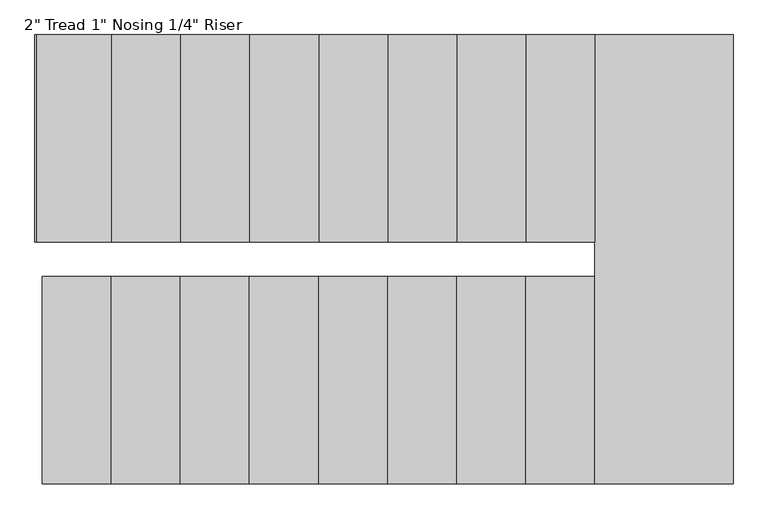
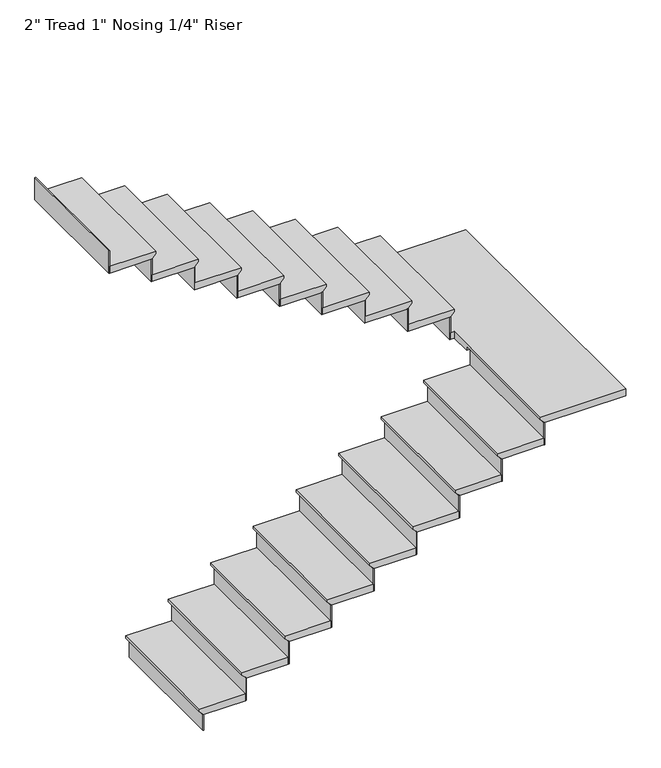
"""IFC4 building model written with IfcOpenShell, lengths in millimetres: stair flight geometry."""

from ifc_helpers import new_model, si_unit, origin, place, context, project, spatial, faceted_brep, source, transform, mapped, element, save


def stair_flight_c80fa3e3(model_context):
    return source(origin(), model_context, "Body", "Brep", [
        faceted_brep([(-1197.97188, -4816.50869, 12799.4833333), (-1197.97188, -4816.50869, 12818.5333333), (-1197.97188, -3902.10869, 12818.5333333), (-1197.97188, -3902.10869, 12799.4833333), (-1172.57188, -4816.50869, 12774.0833333), (-1172.57188, -3902.10869, 12774.0833333), (-867.77188, -4816.50869, 12818.5333333), (-867.77188, -3902.10869, 12818.5333333), (-1172.57188, -3902.10869, 12767.7333333), (-867.77188, -3902.10869, 12767.7333333), (-867.77188, -4816.50869, 12767.7333333), (-1172.57188, -4816.50869, 12767.7333333)], [[[0, 1, 2, 3]], [[4, 0, 3, 5]], [[2, 1, 6, 7]], [[8, 9, 10, 11]], [[2, 7, 9, 8, 5, 3]], [[8, 11, 4, 5]], [[6, 1, 0, 4, 11, 10]], [[7, 6, 10, 9]]]),
        faceted_brep([(-1172.57188, -4816.50869, 12767.7333333), (-1172.57188, -4816.50869, 12649.2), (-1166.22188, -4816.50869, 12649.2), (-1166.22188, -4816.50869, 12767.7333333), (-1172.57188, -3902.10869, 12767.7333333), (-1166.22188, -3902.10869, 12767.7333333), (-1166.22188, -3902.10869, 12649.2), (-1172.57188, -3902.10869, 12649.2)], [[[0, 1, 2, 3]], [[4, 5, 6, 7]], [[1, 0, 4, 7]], [[2, 1, 7, 6]], [[3, 2, 6, 5]], [[0, 3, 5, 4]]]),
        faceted_brep([(-867.77188, -4816.50869, 12937.0666667), (-867.77188, -4816.50869, 12767.7333333), (-861.42188, -4816.50869, 12767.7333333), (-861.42188, -4816.50869, 12937.0666667), (-867.77188, -3902.10869, 12937.0666667), (-861.42188, -3902.10869, 12937.0666667), (-861.42188, -3902.10869, 12767.7333333), (-867.77188, -3902.10869, 12767.7333333)], [[[0, 1, 2, 3]], [[4, 5, 6, 7]], [[1, 0, 4, 7]], [[2, 1, 7, 6]], [[3, 2, 6, 5]], [[0, 3, 5, 4]]]),
        faceted_brep([(-893.17188, -3902.10869, 12987.8666667), (-893.17188, -4816.50869, 12987.8666667), (-562.97188, -4816.50869, 12987.8666667), (-562.97188, -3902.10869, 12987.8666667), (-867.77188, -3902.10869, 12937.0666667), (-562.97188, -3902.10869, 12937.0666667), (-562.97188, -4816.50869, 12937.0666667), (-867.77188, -4816.50869, 12937.0666667), (-867.77188, -3902.10869, 12943.4166667), (-893.17188, -3902.10869, 12968.8166667), (-867.77188, -4816.50869, 12943.4166667), (-893.17188, -4816.50869, 12968.8166667)], [[[0, 1, 2, 3]], [[4, 5, 6, 7]], [[0, 3, 5, 4, 8, 9]], [[4, 7, 10, 8]], [[2, 1, 11, 10, 7, 6]], [[3, 2, 6, 5]], [[11, 1, 0, 9]], [[10, 11, 9, 8]]]),
        faceted_brep([(-562.97188, -4816.50869, 13106.4), (-562.97188, -4816.50869, 12937.0666667), (-556.62188, -4816.50869, 12937.0666667), (-556.62188, -4816.50869, 13106.4), (-562.97188, -3902.10869, 13106.4), (-556.62188, -3902.10869, 13106.4), (-556.62188, -3902.10869, 12937.0666667), (-562.97188, -3902.10869, 12937.0666667)], [[[0, 1, 2, 3]], [[4, 5, 6, 7]], [[1, 0, 4, 7]], [[2, 1, 7, 6]], [[3, 2, 6, 5]], [[0, 3, 5, 4]]]),
        faceted_brep([(-588.37188, -3902.10869, 13157.2), (-588.37188, -4816.50869, 13157.2), (-258.17188, -4816.50869, 13157.2), (-258.17188, -3902.10869, 13157.2), (-562.97188, -3902.10869, 13106.4), (-258.17188, -3902.10869, 13106.4), (-258.17188, -4816.50869, 13106.4), (-562.97188, -4816.50869, 13106.4), (-562.97188, -3902.10869, 13112.75), (-588.37188, -3902.10869, 13138.15), (-562.97188, -4816.50869, 13112.75), (-588.37188, -4816.50869, 13138.15)], [[[0, 1, 2, 3]], [[4, 5, 6, 7]], [[0, 3, 5, 4, 8, 9]], [[4, 7, 10, 8]], [[2, 1, 11, 10, 7, 6]], [[3, 2, 6, 5]], [[11, 1, 0, 9]], [[10, 11, 9, 8]]]),
        faceted_brep([(-258.17188, -4816.50869, 13275.7333333), (-258.17188, -4816.50869, 13106.4), (-251.82188, -4816.50869, 13106.4), (-251.82188, -4816.50869, 13275.7333333), (-258.17188, -3902.10869, 13275.7333333), (-251.82188, -3902.10869, 13275.7333333), (-251.82188, -3902.10869, 13106.4), (-258.17188, -3902.10869, 13106.4)], [[[0, 1, 2, 3]], [[4, 5, 6, 7]], [[1, 0, 4, 7]], [[2, 1, 7, 6]], [[3, 2, 6, 5]], [[0, 3, 5, 4]]]),
        faceted_brep([(-283.57188, -3902.10869, 13326.5333333), (-283.57188, -4816.50869, 13326.5333333), (46.62812, -4816.50869, 13326.5333333), (46.62812, -3902.10869, 13326.5333333), (-258.17188, -3902.10869, 13275.7333333), (46.62812, -3902.10869, 13275.7333333), (46.62812, -4816.50869, 13275.7333333), (-258.17188, -4816.50869, 13275.7333333), (-258.17188, -3902.10869, 13282.0833333), (-283.57188, -3902.10869, 13307.4833333), (-258.17188, -4816.50869, 13282.0833333), (-283.57188, -4816.50869, 13307.4833333)], [[[0, 1, 2, 3]], [[4, 5, 6, 7]], [[0, 3, 5, 4, 8, 9]], [[4, 7, 10, 8]], [[2, 1, 11, 10, 7, 6]], [[3, 2, 6, 5]], [[11, 1, 0, 9]], [[10, 11, 9, 8]]]),
        faceted_brep([(46.62812, -4816.50869, 13445.0666667), (46.62812, -4816.50869, 13275.7333333), (52.97812, -4816.50869, 13275.7333333), (52.97812, -4816.50869, 13445.0666667), (46.62812, -3902.10869, 13445.0666667), (52.97812, -3902.10869, 13445.0666667), (52.97812, -3902.10869, 13275.7333333), (46.62812, -3902.10869, 13275.7333333)], [[[0, 1, 2, 3]], [[4, 5, 6, 7]], [[1, 0, 4, 7]], [[2, 1, 7, 6]], [[3, 2, 6, 5]], [[0, 3, 5, 4]]]),
        faceted_brep([(21.22812, -3902.10869, 13495.8666667), (21.22812, -4816.50869, 13495.8666667), (351.42812, -4816.50869, 13495.8666667), (351.42812, -3902.10869, 13495.8666667), (46.62812, -3902.10869, 13445.0666667), (351.42812, -3902.10869, 13445.0666667), (351.42812, -4816.50869, 13445.0666667), (46.62812, -4816.50869, 13445.0666667), (46.62812, -3902.10869, 13451.4166667), (21.22812, -3902.10869, 13476.8166667), (46.62812, -4816.50869, 13451.4166667), (21.22812, -4816.50869, 13476.8166667)], [[[0, 1, 2, 3]], [[4, 5, 6, 7]], [[0, 3, 5, 4, 8, 9]], [[4, 7, 10, 8]], [[2, 1, 11, 10, 7, 6]], [[3, 2, 6, 5]], [[11, 1, 0, 9]], [[10, 11, 9, 8]]]),
        faceted_brep([(351.42812, -4816.50869, 13614.4), (351.42812, -4816.50869, 13445.0666667), (357.77812, -4816.50869, 13445.0666667), (357.77812, -4816.50869, 13614.4), (351.42812, -3902.10869, 13614.4), (357.77812, -3902.10869, 13614.4), (357.77812, -3902.10869, 13445.0666667), (351.42812, -3902.10869, 13445.0666667)], [[[0, 1, 2, 3]], [[4, 5, 6, 7]], [[1, 0, 4, 7]], [[2, 1, 7, 6]], [[3, 2, 6, 5]], [[0, 3, 5, 4]]]),
        faceted_brep([(326.02812, -3902.10869, 13665.2), (326.02812, -4816.50869, 13665.2), (656.22812, -4816.50869, 13665.2), (656.22812, -3902.10869, 13665.2), (351.42812, -3902.10869, 13614.4), (656.22812, -3902.10869, 13614.4), (656.22812, -4816.50869, 13614.4), (351.42812, -4816.50869, 13614.4), (351.42812, -3902.10869, 13620.75), (326.02812, -3902.10869, 13646.15), (351.42812, -4816.50869, 13620.75), (326.02812, -4816.50869, 13646.15)], [[[0, 1, 2, 3]], [[4, 5, 6, 7]], [[0, 3, 5, 4, 8, 9]], [[4, 7, 10, 8]], [[2, 1, 11, 10, 7, 6]], [[3, 2, 6, 5]], [[11, 1, 0, 9]], [[10, 11, 9, 8]]]),
        faceted_brep([(656.22812, -4816.50869, 13783.7333333), (656.22812, -4816.50869, 13614.4), (662.57812, -4816.50869, 13614.4), (662.57812, -4816.50869, 13783.7333333), (656.22812, -3902.10869, 13783.7333333), (662.57812, -3902.10869, 13783.7333333), (662.57812, -3902.10869, 13614.4), (656.22812, -3902.10869, 13614.4)], [[[0, 1, 2, 3]], [[4, 5, 6, 7]], [[1, 0, 4, 7]], [[2, 1, 7, 6]], [[3, 2, 6, 5]], [[0, 3, 5, 4]]]),
        faceted_brep([(630.82812, -3902.10869, 13834.5333333), (630.82812, -4816.50869, 13834.5333333), (961.02812, -4816.50869, 13834.5333333), (961.02812, -3902.10869, 13834.5333333), (656.22812, -3902.10869, 13783.7333333), (961.02812, -3902.10869, 13783.7333333), (961.02812, -4816.50869, 13783.7333333), (656.22812, -4816.50869, 13783.7333333), (656.22812, -3902.10869, 13790.0833333), (630.82812, -3902.10869, 13815.4833333), (656.22812, -4816.50869, 13790.0833333), (630.82812, -4816.50869, 13815.4833333)], [[[0, 1, 2, 3]], [[4, 5, 6, 7]], [[0, 3, 5, 4, 8, 9]], [[4, 7, 10, 8]], [[2, 1, 11, 10, 7, 6]], [[3, 2, 6, 5]], [[11, 1, 0, 9]], [[10, 11, 9, 8]]]),
        faceted_brep([(961.02812, -4816.50869, 13953.0666667), (961.02812, -4816.50869, 13783.7333333), (967.37812, -4816.50869, 13783.7333333), (967.37812, -4816.50869, 13953.0666667), (961.02812, -3902.10869, 13953.0666667), (967.37812, -3902.10869, 13953.0666667), (967.37812, -3902.10869, 13783.7333333), (961.02812, -3902.10869, 13783.7333333)], [[[0, 1, 2, 3]], [[4, 5, 6, 7]], [[1, 0, 4, 7]], [[2, 1, 7, 6]], [[3, 2, 6, 5]], [[0, 3, 5, 4]]]),
        faceted_brep([(935.62812, -3902.10869, 14003.8666667), (935.62812, -4816.50869, 14003.8666667), (1265.82812, -4816.50869, 14003.8666667), (1265.82812, -3902.10869, 14003.8666667), (961.02812, -3902.10869, 13953.0666667), (1265.82812, -3902.10869, 13953.0666667), (1265.82812, -4816.50869, 13953.0666667), (961.02812, -4816.50869, 13953.0666667), (961.02812, -3902.10869, 13959.4166667), (935.62812, -3902.10869, 13984.8166667), (961.02812, -4816.50869, 13959.4166667), (935.62812, -4816.50869, 13984.8166667)], [[[0, 1, 2, 3]], [[4, 5, 6, 7]], [[0, 3, 5, 4, 8, 9]], [[4, 7, 10, 8]], [[2, 1, 11, 10, 7, 6]], [[3, 2, 6, 5]], [[11, 1, 0, 9]], [[10, 11, 9, 8]]]),
        faceted_brep([(1265.82812, -4816.50869, 14122.4), (1265.82812, -4816.50869, 13953.0666667), (1272.17812, -4816.50869, 13953.0666667), (1272.17812, -4816.50869, 14122.4), (1265.82812, -3902.10869, 14122.4), (1272.17812, -3902.10869, 14122.4), (1272.17812, -3902.10869, 13953.0666667), (1265.82812, -3902.10869, 13953.0666667)], [[[0, 1, 2, 3]], [[4, 5, 6, 7]], [[1, 0, 4, 7]], [[2, 1, 7, 6]], [[3, 2, 6, 5]], [[0, 3, 5, 4]]]),
        faceted_brep([(1215.02812, -3749.70869, 14173.2), (1240.42812, -3749.70869, 14173.2), (1240.42812, -4816.50869, 14173.2), (1850.02812, -4816.50869, 14173.2), (1850.02812, -2835.30869, 14173.2), (1215.02812, -2835.30869, 14173.2), (1240.42812, -3749.70869, 14122.4), (1215.02812, -3749.70869, 14122.4), (1215.02812, -2835.30869, 14122.4), (1850.02812, -2835.30869, 14122.4), (1850.02812, -4816.50869, 14122.4), (1265.82812, -4816.50869, 14122.4), (1265.82812, -3902.10869, 14122.4), (1240.42812, -3902.10869, 14122.4), (1240.42812, -3902.10869, 14154.15), (1240.42812, -4816.50869, 14154.15), (1265.82812, -3902.10869, 14128.75), (1265.82812, -4816.50869, 14128.75)], [[[0, 1, 2, 3, 4, 5]], [[6, 7, 8, 9, 10, 11, 12, 13]], [[1, 0, 7, 6]], [[2, 1, 6, 13, 14, 15]], [[13, 12, 16, 14]], [[12, 11, 17, 16]], [[3, 2, 15, 17, 11, 10]], [[4, 3, 10, 9]], [[5, 4, 9, 8]], [[0, 5, 8, 7]], [[17, 15, 14, 16]]]),
        faceted_brep([(1215.02812, -2835.30869, 14291.7333333), (1215.02812, -2835.30869, 14122.4), (1208.67812, -2835.30869, 14122.4), (1208.67812, -2835.30869, 14291.7333333), (1215.02812, -3749.70869, 14291.7333333), (1208.67812, -3749.70869, 14291.7333333), (1208.67812, -3749.70869, 14122.4), (1215.02812, -3749.70869, 14122.4)], [[[0, 1, 2, 3]], [[4, 5, 6, 7]], [[1, 0, 4, 7]], [[2, 1, 7, 6]], [[3, 2, 6, 5]], [[0, 3, 5, 4]]]),
        faceted_brep([(1240.42812, -3749.70869, 14342.5333333), (1240.42812, -2835.30869, 14342.5333333), (910.22812, -2835.30869, 14342.5333333), (910.22812, -3749.70869, 14342.5333333), (1215.02812, -3749.70869, 14291.7333333), (910.22812, -3749.70869, 14291.7333333), (910.22812, -2835.30869, 14291.7333333), (1215.02812, -2835.30869, 14291.7333333), (1215.02812, -3749.70869, 14298.0833333), (1240.42812, -3749.70869, 14323.4833333), (1215.02812, -2835.30869, 14298.0833333), (1240.42812, -2835.30869, 14323.4833333)], [[[0, 1, 2, 3]], [[4, 5, 6, 7]], [[0, 3, 5, 4, 8, 9]], [[4, 7, 10, 8]], [[2, 1, 11, 10, 7, 6]], [[3, 2, 6, 5]], [[11, 1, 0, 9]], [[10, 11, 9, 8]]]),
        faceted_brep([(910.22812, -2835.30869, 14461.0666667), (910.22812, -2835.30869, 14291.7333333), (903.87812, -2835.30869, 14291.7333333), (903.87812, -2835.30869, 14461.0666667), (910.22812, -3749.70869, 14461.0666667), (903.87812, -3749.70869, 14461.0666667), (903.87812, -3749.70869, 14291.7333333), (910.22812, -3749.70869, 14291.7333333)], [[[0, 1, 2, 3]], [[4, 5, 6, 7]], [[1, 0, 4, 7]], [[2, 1, 7, 6]], [[3, 2, 6, 5]], [[0, 3, 5, 4]]]),
        faceted_brep([(935.62812, -3749.70869, 14511.8666667), (935.62812, -2835.30869, 14511.8666667), (605.42812, -2835.30869, 14511.8666667), (605.42812, -3749.70869, 14511.8666667), (910.22812, -3749.70869, 14461.0666667), (605.42812, -3749.70869, 14461.0666667), (605.42812, -2835.30869, 14461.0666667), (910.22812, -2835.30869, 14461.0666667), (910.22812, -3749.70869, 14467.4166667), (935.62812, -3749.70869, 14492.8166667), (910.22812, -2835.30869, 14467.4166667), (935.62812, -2835.30869, 14492.8166667)], [[[0, 1, 2, 3]], [[4, 5, 6, 7]], [[0, 3, 5, 4, 8, 9]], [[4, 7, 10, 8]], [[2, 1, 11, 10, 7, 6]], [[3, 2, 6, 5]], [[11, 1, 0, 9]], [[10, 11, 9, 8]]]),
        faceted_brep([(605.42812, -2835.30869, 14630.4), (605.42812, -2835.30869, 14461.0666667), (599.07812, -2835.30869, 14461.0666667), (599.07812, -2835.30869, 14630.4), (605.42812, -3749.70869, 14630.4), (599.07812, -3749.70869, 14630.4), (599.07812, -3749.70869, 14461.0666667), (605.42812, -3749.70869, 14461.0666667)], [[[0, 1, 2, 3]], [[4, 5, 6, 7]], [[1, 0, 4, 7]], [[2, 1, 7, 6]], [[3, 2, 6, 5]], [[0, 3, 5, 4]]]),
        faceted_brep([(630.82812, -3749.70869, 14681.2), (630.82812, -2835.30869, 14681.2), (300.62812, -2835.30869, 14681.2), (300.62812, -3749.70869, 14681.2), (605.42812, -3749.70869, 14630.4), (300.62812, -3749.70869, 14630.4), (300.62812, -2835.30869, 14630.4), (605.42812, -2835.30869, 14630.4), (605.42812, -3749.70869, 14636.75), (630.82812, -3749.70869, 14662.15), (605.42812, -2835.30869, 14636.75), (630.82812, -2835.30869, 14662.15)], [[[0, 1, 2, 3]], [[4, 5, 6, 7]], [[0, 3, 5, 4, 8, 9]], [[4, 7, 10, 8]], [[2, 1, 11, 10, 7, 6]], [[3, 2, 6, 5]], [[11, 1, 0, 9]], [[10, 11, 9, 8]]]),
        faceted_brep([(300.62812, -2835.30869, 14799.7333333), (300.62812, -2835.30869, 14630.4), (294.27812, -2835.30869, 14630.4), (294.27812, -2835.30869, 14799.7333333), (300.62812, -3749.70869, 14799.7333333), (294.27812, -3749.70869, 14799.7333333), (294.27812, -3749.70869, 14630.4), (300.62812, -3749.70869, 14630.4)], [[[0, 1, 2, 3]], [[4, 5, 6, 7]], [[1, 0, 4, 7]], [[2, 1, 7, 6]], [[3, 2, 6, 5]], [[0, 3, 5, 4]]]),
        faceted_brep([(326.02812, -3749.70869, 14850.5333333), (326.02812, -2835.30869, 14850.5333333), (-4.17188, -2835.30869, 14850.5333333), (-4.17188, -3749.70869, 14850.5333333), (300.62812, -3749.70869, 14799.7333333), (-4.17188, -3749.70869, 14799.7333333), (-4.17188, -2835.30869, 14799.7333333), (300.62812, -2835.30869, 14799.7333333), (300.62812, -3749.70869, 14806.0833333), (326.02812, -3749.70869, 14831.4833333), (300.62812, -2835.30869, 14806.0833333), (326.02812, -2835.30869, 14831.4833333)], [[[0, 1, 2, 3]], [[4, 5, 6, 7]], [[0, 3, 5, 4, 8, 9]], [[4, 7, 10, 8]], [[2, 1, 11, 10, 7, 6]], [[3, 2, 6, 5]], [[11, 1, 0, 9]], [[10, 11, 9, 8]]]),
        faceted_brep([(-4.17188, -2835.30869, 14969.0666667), (-4.17188, -2835.30869, 14799.7333333), (-10.52188, -2835.30869, 14799.7333333), (-10.52188, -2835.30869, 14969.0666667), (-4.17188, -3749.70869, 14969.0666667), (-10.52188, -3749.70869, 14969.0666667), (-10.52188, -3749.70869, 14799.7333333), (-4.17188, -3749.70869, 14799.7333333)], [[[0, 1, 2, 3]], [[4, 5, 6, 7]], [[1, 0, 4, 7]], [[2, 1, 7, 6]], [[3, 2, 6, 5]], [[0, 3, 5, 4]]]),
        faceted_brep([(21.22812, -3749.70869, 15019.8666667), (21.22812, -2835.30869, 15019.8666667), (-308.97188, -2835.30869, 15019.8666667), (-308.97188, -3749.70869, 15019.8666667), (-4.17188, -3749.70869, 14969.0666667), (-308.97188, -3749.70869, 14969.0666667), (-308.97188, -2835.30869, 14969.0666667), (-4.17188, -2835.30869, 14969.0666667), (-4.17188, -3749.70869, 14975.4166667), (21.22812, -3749.70869, 15000.8166667), (-4.17188, -2835.30869, 14975.4166667), (21.22812, -2835.30869, 15000.8166667)], [[[0, 1, 2, 3]], [[4, 5, 6, 7]], [[0, 3, 5, 4, 8, 9]], [[4, 7, 10, 8]], [[2, 1, 11, 10, 7, 6]], [[3, 2, 6, 5]], [[11, 1, 0, 9]], [[10, 11, 9, 8]]]),
        faceted_brep([(-308.97188, -2835.30869, 15138.4), (-308.97188, -2835.30869, 14969.0666667), (-315.32188, -2835.30869, 14969.0666667), (-315.32188, -2835.30869, 15138.4), (-308.97188, -3749.70869, 15138.4), (-315.32188, -3749.70869, 15138.4), (-315.32188, -3749.70869, 14969.0666667), (-308.97188, -3749.70869, 14969.0666667)], [[[0, 1, 2, 3]], [[4, 5, 6, 7]], [[1, 0, 4, 7]], [[2, 1, 7, 6]], [[3, 2, 6, 5]], [[0, 3, 5, 4]]]),
        faceted_brep([(-283.57188, -3749.70869, 15189.2), (-283.57188, -2835.30869, 15189.2), (-613.77188, -2835.30869, 15189.2), (-613.77188, -3749.70869, 15189.2), (-308.97188, -3749.70869, 15138.4), (-613.77188, -3749.70869, 15138.4), (-613.77188, -2835.30869, 15138.4), (-308.97188, -2835.30869, 15138.4), (-308.97188, -3749.70869, 15144.75), (-283.57188, -3749.70869, 15170.15), (-308.97188, -2835.30869, 15144.75), (-283.57188, -2835.30869, 15170.15)], [[[0, 1, 2, 3]], [[4, 5, 6, 7]], [[0, 3, 5, 4, 8, 9]], [[4, 7, 10, 8]], [[2, 1, 11, 10, 7, 6]], [[3, 2, 6, 5]], [[11, 1, 0, 9]], [[10, 11, 9, 8]]]),
        faceted_brep([(-613.77188, -2835.30869, 15307.7333333), (-613.77188, -2835.30869, 15138.4), (-620.12188, -2835.30869, 15138.4), (-620.12188, -2835.30869, 15307.7333333), (-613.77188, -3749.70869, 15307.7333333), (-620.12188, -3749.70869, 15307.7333333), (-620.12188, -3749.70869, 15138.4), (-613.77188, -3749.70869, 15138.4)], [[[0, 1, 2, 3]], [[4, 5, 6, 7]], [[1, 0, 4, 7]], [[2, 1, 7, 6]], [[3, 2, 6, 5]], [[0, 3, 5, 4]]]),
        faceted_brep([(-588.37188, -3749.70869, 15358.5333333), (-588.37188, -2835.30869, 15358.5333333), (-918.57188, -2835.30869, 15358.5333333), (-918.57188, -3749.70869, 15358.5333333), (-613.77188, -3749.70869, 15307.7333333), (-918.57188, -3749.70869, 15307.7333333), (-918.57188, -2835.30869, 15307.7333333), (-613.77188, -2835.30869, 15307.7333333), (-613.77188, -3749.70869, 15314.0833333), (-588.37188, -3749.70869, 15339.4833333), (-613.77188, -2835.30869, 15314.0833333), (-588.37188, -2835.30869, 15339.4833333)], [[[0, 1, 2, 3]], [[4, 5, 6, 7]], [[0, 3, 5, 4, 8, 9]], [[4, 7, 10, 8]], [[2, 1, 11, 10, 7, 6]], [[3, 2, 6, 5]], [[11, 1, 0, 9]], [[10, 11, 9, 8]]]),
        faceted_brep([(-918.57188, -2835.30869, 15477.0666667), (-918.57188, -2835.30869, 15307.7333333), (-924.92188, -2835.30869, 15307.7333333), (-924.92188, -2835.30869, 15477.0666667), (-918.57188, -3749.70869, 15477.0666667), (-924.92188, -3749.70869, 15477.0666667), (-924.92188, -3749.70869, 15307.7333333), (-918.57188, -3749.70869, 15307.7333333)], [[[0, 1, 2, 3]], [[4, 5, 6, 7]], [[1, 0, 4, 7]], [[2, 1, 7, 6]], [[3, 2, 6, 5]], [[0, 3, 5, 4]]]),
        faceted_brep([(-1223.37188, -2835.30869, 15646.4), (-1223.37188, -2835.30869, 15477.0666667), (-1229.72188, -2835.30869, 15477.0666667), (-1229.72188, -2835.30869, 15646.4), (-1223.37188, -3749.70869, 15646.4), (-1229.72188, -3749.70869, 15646.4), (-1229.72188, -3749.70869, 15477.0666667), (-1223.37188, -3749.70869, 15477.0666667)], [[[0, 1, 2, 3]], [[4, 5, 6, 7]], [[1, 0, 4, 7]], [[2, 1, 7, 6]], [[3, 2, 6, 5]], [[0, 3, 5, 4]]]),
        faceted_brep([(-893.17188, -3749.70869, 15527.8666667), (-893.17188, -2835.30869, 15527.8666667), (-1223.37188, -2835.30869, 15527.8666667), (-1223.37188, -3749.70869, 15527.8666667), (-918.57188, -3749.70869, 15477.0666667), (-1223.37188, -3749.70869, 15477.0666667), (-1223.37188, -2835.30869, 15477.0666667), (-918.57188, -2835.30869, 15477.0666667), (-918.57188, -3749.70869, 15483.4166667), (-893.17188, -3749.70869, 15508.8166667), (-918.57188, -2835.30869, 15483.4166667), (-893.17188, -2835.30869, 15508.8166667)], [[[0, 1, 2, 3]], [[4, 5, 6, 7]], [[0, 3, 5, 4, 8, 9]], [[4, 7, 10, 8]], [[2, 1, 11, 10, 7, 6]], [[3, 2, 6, 5]], [[11, 1, 0, 9]], [[10, 11, 9, 8]]]),
    ])


if __name__ == "__main__":
    model = new_model("IFC4")
    model_context = context("Model", 3, world=origin())
    ifc_project = project(units=[si_unit("LENGTHUNIT", "METRE", prefix="MILLI")], contexts=[model_context])
    site = spatial("IfcSite", under=ifc_project)
    building = spatial("IfcBuilding", under=site)
    placement = place(None, origin())
    stair_flight_shape = stair_flight_c80fa3e3(model_context)
    element("IfcStairFlight", 1, ObjectType="2\" Tread 1\" Nosing 1/4\" Riser", at=placement, inside=building, context=model_context, shape_type="MappedRepresentation", body=[
        mapped(stair_flight_shape, transform((0.0, 0.0, 0.0), x_axis=(1.0, 0.0, 0.0), y_axis=(0.0, 1.0, 0.0), z_axis=(0.0, 0.0, 1.0))),
    ])
    save(model, "model.ifc")
